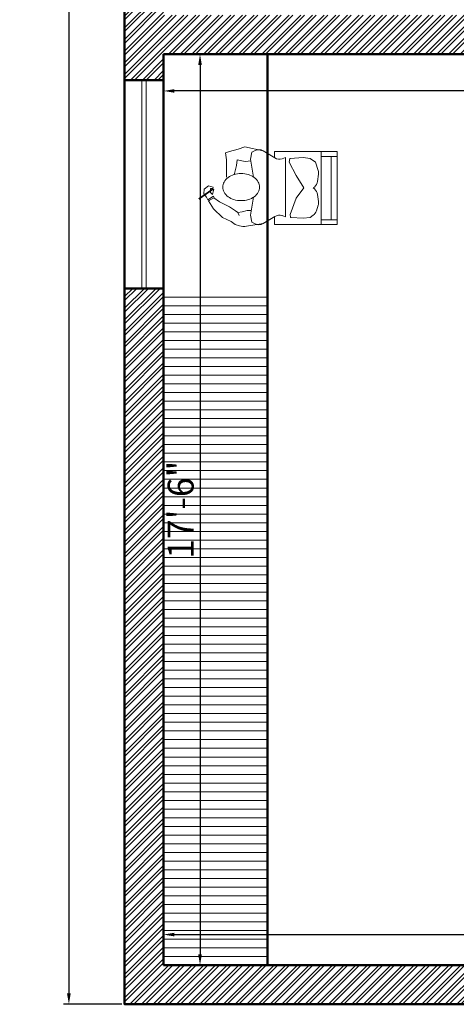
# Model space of a CAD drawing. Units: inches. Extents: x 3590 to 5167, y 65 to 1917.
# Tile 7 of 100: x 4396 to 4497, y 109 to 336. Entities that reach past the tile are written whole.
import ezdxf

# ---------------------------------------------------------------- set-up
doc = ezdxf.new("R2010")
doc.units = ezdxf.units.IN
for name, color, linetype, lineweight in [('A-ANNO-DIMS', 2, 'Continuous', 18), ('A-FURN', 21, 'Continuous', 18), ('A-GLAZ', 4, 'Continuous', 18), ('A-WALL', 7, 'Continuous', 50), ('A-WALL-PATT', 251, 'Continuous', 13)]:
    doc.layers.add(name, color=color, linetype=linetype, lineweight=lineweight)
doc.styles.get("Standard").update_dxf_attribs({"font": 'arial.ttf'})
doc.dimstyles.new('ISO-25', dxfattribs={"dimtxt": 9, "dimasz": 2.5, "dimexe": 1.25, "dimexo": 0.625, "dimtad": 1, "dimdec": 1, "dimlunit": 3, "dimtxsty": 'Standard', "dimcen": 2.5, "dimadec": 0, "dimazin": 0, "dimtfac": 1, "dimtdec": 1, "dimtmove": 0, "dimatfit": 3, "dimfxl": 1, "dimarcsym": 0})

# ---------------------------------------------------------------- blocks, each defined once
blk = doc.blocks.new('*D280')
at = {"layer": 'A-ANNO-DIMS', "color": 0, "lineweight": -2, "transparency": 16777216}
for p, q in [((4419.65, 589.06), (4406.15, 589.06)), ((4407.4, 586.56), (4407.4, 111.56)), ((4419.65, 109.06), (4406.15, 109.06))]:
    blk.add_line(p, q, dxfattribs=at)
at = {"layer": 'A-ANNO-DIMS', "color": 0, "transparency": 16777216}
for points in [[(4406.98, 586.56), (4407.82, 586.56), (4407.4, 589.06)], [(4406.98, 111.56), (4407.82, 111.56), (4407.4, 109.06)]]:
    blk.add_solid(points, dxfattribs=at)
at = {"layer": 'Defpoints', "color": 0, "transparency": 16777216}
for p in [(4420.27, 589.06), (4407.4, 109.06), (4420.27, 109.06)]:
    blk.add_point(p, dxfattribs=at)
at = {"layer": 'A-ANNO-DIMS', "color": 0, "transparency": 16777216, "insert": (4402.18, 349.06), "char_height": 9, "attachment_point": 5, "rotation": 90}
blk.add_mtext("40'", dxfattribs=at)
blk = doc.blocks.new('*D265')
at = {"layer": 'A-ANNO-DIMS', "color": 0, "lineweight": -2, "transparency": 16777216}
for p, q in [((4429.27, 327.43), (4429.27, 318.33)), ((4639.27, 327.43), (4639.27, 318.33)), ((4636.77, 319.58), (4431.77, 319.58))]:
    blk.add_line(p, q, dxfattribs=at)
at = {"layer": 'A-ANNO-DIMS', "color": 0, "transparency": 16777216}
for points in [[(4431.77, 319.99), (4431.77, 319.16), (4429.27, 319.58)], [(4636.77, 319.99), (4636.77, 319.16), (4639.27, 319.58)]]:
    blk.add_solid(points, dxfattribs=at)
at = {"layer": 'Defpoints', "color": 0, "transparency": 16777216}
for p in [(4429.27, 328.06), (4639.27, 328.06), (4429.27, 319.58)]:
    blk.add_point(p, dxfattribs=at)
at = {"layer": 'A-ANNO-DIMS', "color": 0, "transparency": 16777216, "insert": (4534.27, 323.26), "char_height": 6, "attachment_point": 5}
blk.add_mtext('17\'-6"', dxfattribs=at)
blk = doc.blocks.new('*D224')
at = {"layer": 'A-ANNO-DIMS', "color": 0, "lineweight": -2, "transparency": 16777216}
for p, q in [((4429.9, 328.06), (4438.92, 328.06)), ((4437.67, 325.56), (4437.67, 120.56)), ((4429.9, 118.06), (4438.92, 118.06))]:
    blk.add_line(p, q, dxfattribs=at)
at = {"layer": 'A-ANNO-DIMS', "color": 0, "transparency": 16777216}
for points in [[(4437.25, 325.56), (4438.08, 325.56), (4437.67, 328.06)], [(4437.25, 120.56), (4438.08, 120.56), (4437.67, 118.06)]]:
    blk.add_solid(points, dxfattribs=at)
at = {"layer": 'Defpoints', "color": 0, "transparency": 16777216}
for p in [(4429.27, 328.06), (4429.27, 118.06), (4437.67, 118.06)]:
    blk.add_point(p, dxfattribs=at)
at = {"layer": 'A-ANNO-DIMS', "color": 0, "transparency": 16777216, "insert": (4433.98, 223.06), "char_height": 6, "attachment_point": 5, "rotation": 90}
blk.add_mtext('17\'-6"', dxfattribs=at)
blk = doc.blocks.new('*D225')
at = {"layer": 'A-ANNO-DIMS', "color": 0, "lineweight": -2, "transparency": 16777216}
for p, q in [((4429.27, 118.68), (4429.27, 126.38)), ((4431.77, 125.13), (4636.77, 125.13)), ((4639.27, 118.68), (4639.27, 126.38))]:
    blk.add_line(p, q, dxfattribs=at)
at = {"layer": 'A-ANNO-DIMS', "color": 0, "transparency": 16777216}
for points in [[(4431.77, 125.55), (4431.77, 124.71), (4429.27, 125.13)], [(4636.77, 125.55), (4636.77, 124.71), (4639.27, 125.13)]]:
    blk.add_solid(points, dxfattribs=at)
at = {"layer": 'Defpoints', "color": 0, "transparency": 16777216}
for p in [(4639.27, 125.13), (4429.27, 118.06), (4639.27, 118.06)]:
    blk.add_point(p, dxfattribs=at)
at = {"layer": 'A-ANNO-DIMS', "color": 0, "transparency": 16777216, "insert": (4534.27, 128.82), "char_height": 6, "attachment_point": 5}
blk.add_mtext('17\'-6"', dxfattribs=at)
blk = doc.blocks.new('DESK-CHAIR')
for p, q in [((3674.9, 1522.4), (3674.54, 1520.79)), ((3674.54, 1520.79), (3675.25, 1516.67)), ((3675.51, 1522.74), (3674.9, 1522.4)), ((3680.2, 1521.08), (3677.49, 1522.71)), ((3694.59, 1522.58), (3680.09, 1522.58)), ((3680.09, 1522.58), (3680.09, 1521.15)), ((3682.6, 1521.15), (3681.85, 1520.9)), ((3682.6, 1521.15), (3682.6, 1507.53)), ((3682.6, 1507.53), (3682.6, 1521.15)), ((3683.49, 1520.07), (3683.66, 1520.91)), ((3683.73, 1520.97), (3686.72, 1521.15)), ((3686.72, 1521.15), (3688.33, 1520.97)), ((3688.33, 1520.97), (3689.58, 1520.07)), ((3694.59, 1505.74), (3694.59, 1522.58)), ((3685.1, 1517.02), (3683.49, 1520.07)), ((3689.58, 1520.07), (3690.17, 1518.15)), ((3686.89, 1514.16), (3685.1, 1517.02)), ((3690.24, 1517.32), (3690.04, 1515.67)), ((3685.1, 1511.83), (3686.89, 1514.16)), ((3689.31, 1514.37), (3689.04, 1514.16)), ((3689.31, 1513.95), (3689.04, 1514.16)), ((3664.74, 1511.43), (3666.04, 1512.26)), ((3665.07, 1511.29), (3664.74, 1511.43)), ((3664.84, 1511.19), (3666.07, 1511.86)), ((3666.04, 1512.26), (3666.24, 1511.79)), ((3666.07, 1511.86), (3667.43, 1510.93)), ((3674.54, 1507.89), (3675.25, 1512.01)), ((3683.67, 1508.07), (3685.1, 1511.83)), ((3690.24, 1511), (3690.04, 1512.64)), ((3666.04, 1509.36), (3664.84, 1511.19)), ((3668.13, 1507.37), (3666.04, 1509.36)), ((3667.43, 1510.93), (3669.7, 1509.83)), ((3669.7, 1509.83), (3671.06, 1508.9)), ((3689.78, 1508.89), (3690.17, 1510.17)), ((3670.06, 1506.4), (3668.13, 1507.37)), ((3671.06, 1508.9), (3671.66, 1508.47)), ((3671.66, 1508.47), (3671.96, 1507.77)), ((3674.9, 1506.27), (3674.54, 1507.89)), ((3680.2, 1507.6), (3677.49, 1505.97)), ((3680.09, 1507.53), (3680.09, 1505.74)), ((3682.6, 1507.53), (3681.85, 1507.78)), ((3683.8, 1507.4), (3683.67, 1508.07)), ((3683.88, 1507.34), (3686.72, 1507.17)), ((3686.72, 1507.17), (3688.33, 1507.35)), ((3688.33, 1507.35), (3689.03, 1507.86)), ((3677.49, 1505.97), (3673.14, 1505.31)), ((3675.51, 1505.94), (3674.9, 1506.27)), ((3680.09, 1505.74), (3694.59, 1505.74))]:
    blk.add_line(p, q)
for points in [[(3677.49, 1522.71), (3673.28, 1523.65), (3671.67, 1523.12), (3669.7, 1522.58), (3668.81, 1522.22), (3668.99, 1520.61), (3668.99, 1519), (3668.99, 1516.67)], [(3664.74, 1511.43), (3664.42, 1512.05), (3663.77, 1512.78), (3663.87, 1513.9), (3664.88, 1514.67), (3665.92, 1514.37), (3665.9, 1514.02), (3665.32, 1514.02), (3665.3, 1513.1), (3665.82, 1512.66), (3666.07, 1513.84)], [(3671.66, 1508.47), (3672.6, 1508.69), (3673.82, 1508.93), (3674.7, 1508.93)], [(3670.06, 1506.4), (3671.04, 1505.75), (3672.02, 1505.46), (3672.8, 1505.31), (3673.24, 1505.31)]]:
    blk.add_lwpolyline(points)
at = {"const_width": 0.39}
blk.add_lwpolyline([(3666.01, 1513.98), (3662.61, 1511.61)], dxfattribs=at)
for centre, radius, start, end in [((3676.47, 1521), 1.98, 59.0235, 119.0669), ((3681.22, 1522.78), 1.98, 239.0235, 288.4436), ((3683.74, 1520.89), 0.0779, 93.3682, 168.6956), ((3683.74, 1520.89), 0.0779, 93.3682, 168.6956), ((3688.27, 1517.56), 1.98, 352.8785, 17.0946), ((3688.07, 1515.92), 1.98, 308.6739, 352.8785), ((3688.07, 1512.4), 1.98, 7.1215, 51.3261), ((3688.27, 1510.75), 1.98, 342.9054, 7.1215), ((3681.22, 1505.89), 1.98, 71.5564, 120.9765), ((3683.88, 1507.42), 0.0779, 191.3044, 266.6318), ((3687.88, 1509.47), 1.98, 305.5514, 342.9054), ((3676.47, 1507.67), 1.98, 240.9331, 300.9765)]:
    blk.add_arc(centre, radius, start, end)

msp = doc.modelspace()

# ---------------------------------------------------------------- hatches: boundary and pattern name
at = {"layer": 'A-WALL-PATT', "transparency": 33554687}
h = msp.add_hatch(dxfattribs=at)
h.set_pattern_fill('ANSI32', color=256, scale=0.2)
h.set_pattern_definition([(45, (0, -1216.9392), (-1.3470384, 1.3470384), []), (45, (0.898, -1216.9392), (-1.3470384, 1.3470384), [])])
h.paths.add_polyline_path([(4684.27, 589.06), (4591.27, 589.06), (4591.27, 580.06), (4639.27, 580.06), (4639.27, 574.06), (4648.27, 574.06), (4648.27, 580.06), (4684.27, 580.06)])
h.paths.add_polyline_path([(4543.27, 589.06), (4420.27, 589.06), (4420.27, 568.06), (4429.27, 568.06), (4429.27, 580.06), (4445.92, 580.06), (4543.27, 580.06)])
h.paths.add_polyline_path([(4828.27, 589.06), (4744.27, 589.06), (4744.27, 580.06), (4828.27, 580.06)])
h.paths.add_polyline_path([(4648.27, 538.06), (4639.27, 538.06), (4639.27, 439.06), (4546.27, 439.06), (4546.27, 433.06), (4549.27, 433.06), (4549.27, 337.06), (4429.27, 337.06), (4429.27, 367.06), (4420.27, 367.06), (4420.27, 322.06), (4429.27, 322.06), (4429.27, 328.06), (4639.27, 328.06), (4639.27, 322.06), (4648.27, 322.06), (4648.27, 343.06), (4639.27, 343.06), (4639.27, 337.06), (4555.27, 337.06), (4555.27, 433.06), (4639.27, 433.06), (4639.27, 373.06), (4648.27, 373.06)])
h.paths.add_polyline_path([(4516.27, 439.06), (4429.27, 439.06), (4429.27, 520.06), (4420.27, 520.06), (4420.27, 403.06), (4429.27, 403.06), (4429.27, 433.06), (4516.27, 433.06)], flags=17)
h.paths.add_polyline_path([(5080.27, 589.06), (4888.27, 589.06), (4888.27, 580.06), (4924.27, 580.06), (4924.27, 538.06), (4933.27, 538.06), (4933.27, 580.06), (5071.27, 580.06), (5071.27, 118.06), (4933.27, 118.06), (4933.27, 349.06), (4924.27, 349.06), (4924.27, 118.06), (4898.77, 118.06), (4898.77, 109.06), (5080.27, 109.06)])
h.paths.add_polyline_path([(4933.27, 502.06), (4924.27, 502.06), (4924.27, 421.06), (4933.27, 421.06)], flags=17)
h.paths.add_polyline_path([(4802.77, 118.06), (4777.27, 118.06), (4777.27, 286.06), (4756.27, 286.06), (4756.27, 277.06), (4768.27, 277.06), (4768.27, 214.06), (4696.27, 214.06), (4696.27, 277.06), (4708.27, 277.06), (4708.27, 286.06), (4639.27, 286.06), (4639.27, 277.06), (4687.27, 277.06), (4687.27, 214.06), (4681.27, 214.06), (4681.27, 205.06), (4768.27, 205.06), (4768.27, 118.06), (4726.27, 118.06), (4726.27, 109.06), (4802.77, 109.06)])
h.paths.add_polyline_path([(4690.27, 118.06), (4648.27, 118.06), (4648.27, 135.93), (4648.27, 205.06), (4651.27, 205.06), (4651.27, 214.06), (4639.27, 214.06), (4639.27, 118.06), (4633.27, 118.06), (4633.27, 109.06), (4690.27, 109.06)])
h.paths.add_polyline_path([(4585.27, 118.06), (4584.72, 118.06), (4429.27, 118.06), (4429.27, 274.06), (4420.27, 274.06), (4420.27, 109.06), (4585.27, 109.06)])

# ---------------------------------------------------------------- linework, layer by layer
at = {"layer": 'A-FURN'}
for p, q in [((4465.6, 288.8), (4465.6, 305.64)), ((4465.6, 304.49), (4469.36, 304.49)), ((4467.92, 289.9), (4467.92, 304.49)), ((4465.6, 289.9), (4469.36, 289.9)), ((4453.27, 272.06), (4429.27, 272.06)), ((4453.27, 270.06), (4429.27, 270.06)), ((4453.27, 268.06), (4429.27, 268.06)), ((4453.27, 266.06), (4429.27, 266.06)), ((4453.27, 264.06), (4429.27, 264.06)), ((4453.27, 262.06), (4429.27, 262.06)), ((4453.27, 260.06), (4429.27, 260.06)), ((4453.27, 258.06), (4429.27, 258.06)), ((4453.27, 256.06), (4429.27, 256.06)), ((4453.27, 254.06), (4429.27, 254.06)), ((4453.27, 252.06), (4429.27, 252.06)), ((4453.27, 250.06), (4429.27, 250.06)), ((4453.27, 248.06), (4429.27, 248.06)), ((4453.27, 246.06), (4429.27, 246.06)), ((4453.27, 244.06), (4429.27, 244.06)), ((4453.27, 242.06), (4429.27, 242.06)), ((4453.27, 240.06), (4429.27, 240.06)), ((4453.27, 238.06), (4429.27, 238.06)), ((4453.27, 236.06), (4429.27, 236.06)), ((4453.27, 234.06), (4429.27, 234.06)), ((4453.27, 232.06), (4429.27, 232.06)), ((4453.27, 230.06), (4429.27, 230.06)), ((4453.27, 228.06), (4429.27, 228.06)), ((4453.27, 226.06), (4429.27, 226.06)), ((4453.27, 224.06), (4429.27, 224.06)), ((4453.27, 222.06), (4429.27, 222.06)), ((4453.27, 220.06), (4429.27, 220.06)), ((4453.27, 218.06), (4429.27, 218.06)), ((4453.27, 216.06), (4429.27, 216.06)), ((4453.27, 214.06), (4429.27, 214.06)), ((4453.27, 212.06), (4429.27, 212.06)), ((4453.27, 210.06), (4429.27, 210.06)), ((4453.27, 208.06), (4429.27, 208.06)), ((4453.27, 206.06), (4429.27, 206.06)), ((4453.27, 204.06), (4429.27, 204.06)), ((4453.27, 202.06), (4429.27, 202.06)), ((4453.27, 200.06), (4429.27, 200.06)), ((4453.27, 198.06), (4429.27, 198.06)), ((4453.27, 196.06), (4429.27, 196.06)), ((4453.27, 194.06), (4429.27, 194.06)), ((4453.27, 192.06), (4429.27, 192.06)), ((4453.27, 190.06), (4429.27, 190.06)), ((4453.27, 188.06), (4429.27, 188.06)), ((4453.27, 186.06), (4429.27, 186.06)), ((4453.27, 184.06), (4429.27, 184.06)), ((4453.27, 182.06), (4429.27, 182.06)), ((4453.27, 180.06), (4429.27, 180.06)), ((4453.27, 178.06), (4429.27, 178.06)), ((4453.27, 176.06), (4429.27, 176.06)), ((4453.27, 174.06), (4429.27, 174.06)), ((4453.27, 172.06), (4429.27, 172.06)), ((4453.27, 170.06), (4429.27, 170.06)), ((4453.27, 168.06), (4429.27, 168.06)), ((4453.27, 166.06), (4429.27, 166.06)), ((4453.27, 164.06), (4429.27, 164.06)), ((4453.27, 162.06), (4429.27, 162.06)), ((4453.27, 160.06), (4429.27, 160.06)), ((4453.27, 158.06), (4429.27, 158.06)), ((4453.27, 156.06), (4429.27, 156.06)), ((4453.27, 154.06), (4429.27, 154.06)), ((4453.27, 152.06), (4429.27, 152.06)), ((4453.27, 150.06), (4429.27, 150.06)), ((4453.27, 148.06), (4429.27, 148.06)), ((4453.27, 146.06), (4429.27, 146.06)), ((4453.27, 144.06), (4429.27, 144.06)), ((4453.27, 142.06), (4429.27, 142.06)), ((4453.27, 140.06), (4429.27, 140.06)), ((4453.27, 138.06), (4429.27, 138.06)), ((4453.27, 136.06), (4429.27, 136.06)), ((4453.27, 134.06), (4429.27, 134.06)), ((4453.27, 132.06), (4429.27, 132.06)), ((4453.27, 130.06), (4429.27, 130.06)), ((4453.27, 128.06), (4429.27, 128.06)), ((4453.27, 126.06), (4429.27, 126.06)), ((4453.27, 126.06), (4429.27, 126.06)), ((4453.27, 124.06), (4429.27, 124.06)), ((4453.27, 122.06), (4429.27, 122.06)), ((4453.27, 120.06), (4429.27, 120.06))]:
    msp.add_line(p, q, dxfattribs=at)
msp.add_lwpolyline([(4445.54, 300.26), (4446.08, 302.41), (4446.26, 303.67), (4448.05, 303.31), (4449.48, 303.49)], dxfattribs=at)
msp.add_lwpolyline([(4447.15, 294.29, 0.07405), (4448.83, 294.54, 0.084801), (4450.16, 295.2, 0.106336), (4451.1, 296.27, 0.128955), (4451.4, 297.41, 0.128955), (4451.1, 298.55, 0.106336), (4450.16, 299.62, 0.084801), (4448.83, 300.28, 0.07405), (4447.15, 300.53, 0.07405), (4445.48, 300.28, 0.084801), (4444.15, 299.62, 0.106336), (4443.21, 298.55, 0.128955), (4442.91, 297.41, 0.128955), (4443.21, 296.27, 0.106336), (4444.15, 295.2, 0.084801), (4445.48, 294.54, 0.07405)], format="xyb", close=True, dxfattribs=at)
at = {"layer": 'A-GLAZ'}
for p, q in [((4424.27, 274.06), (4424.27, 322.06)), ((4425.27, 274.06), (4425.27, 322.06))]:
    msp.add_line(p, q, dxfattribs=at)
at = {"layer": 'A-WALL'}
for p, q in [((4639.27, 328.06), (4429.27, 328.06)), ((4429.27, 118.06), (4429.27, 328.06)), ((4453.27, 118.06), (4453.27, 328.06)), ((4429.27, 322.06), (4420.27, 322.06)), ((4429.27, 274.06), (4420.27, 274.06)), ((4639.27, 118.06), (4429.27, 118.06))]:
    msp.add_line(p, q, dxfattribs=at)
msp.add_lwpolyline([(5080.27, 589.06), (5080.27, 109.06), (4420.27, 109.06), (4420.27, 589.06)], close=True, dxfattribs=at)

# ---------------------------------------------------------------- block references
at = {"layer": 'A-FURN'}
msp.add_blockref('DESK-CHAIR', (774.76, -1216.94), dxfattribs=at)

# ---------------------------------------------------------------- dimensions: what is measured, and where the dimension line sits
at = {"layer": 'A-ANNO-DIMS'}
for base, p1, p2, override, picture, middle in [((4407.4, 109.06), (4420.27, 589.06), (4420.27, 109.06), {"dimclrd": 0, "dimclre": 0, "dimclrt": 0}, '*D280', (4402.18, 349.06)), ((4437.67, 118.06), (4429.27, 328.06), (4429.27, 118.06), {"dimtxt": 6, "dimclrd": 0, "dimclre": 0, "dimclrt": 0}, '*D224', (4433.98, 223.06))]:
    dim = msp.add_linear_dim(base=base, p1=p1, p2=p2, angle=90, dimstyle='ISO-25', override=override, dxfattribs=at)
    dim.commit()
    dim.dimension.update_dxf_attribs({"geometry": picture, "text_midpoint": middle})
for base, p1, p2, picture, middle in [((4429.27, 319.58), (4639.27, 328.06), (4429.27, 328.06), '*D265', (4534.27, 323.26)), ((4639.27, 125.13), (4429.27, 118.06), (4639.27, 118.06), '*D225', (4534.27, 128.82))]:
    dim = msp.add_linear_dim(base=base, p1=p1, p2=p2, dimstyle='ISO-25', override={"dimtxt": 6, "dimclrd": 0, "dimclre": 0, "dimclrt": 0}, dxfattribs=at)
    dim.commit()
    dim.dimension.update_dxf_attribs({"geometry": picture, "text_midpoint": middle})

doc.saveas('drawing.dxf')
